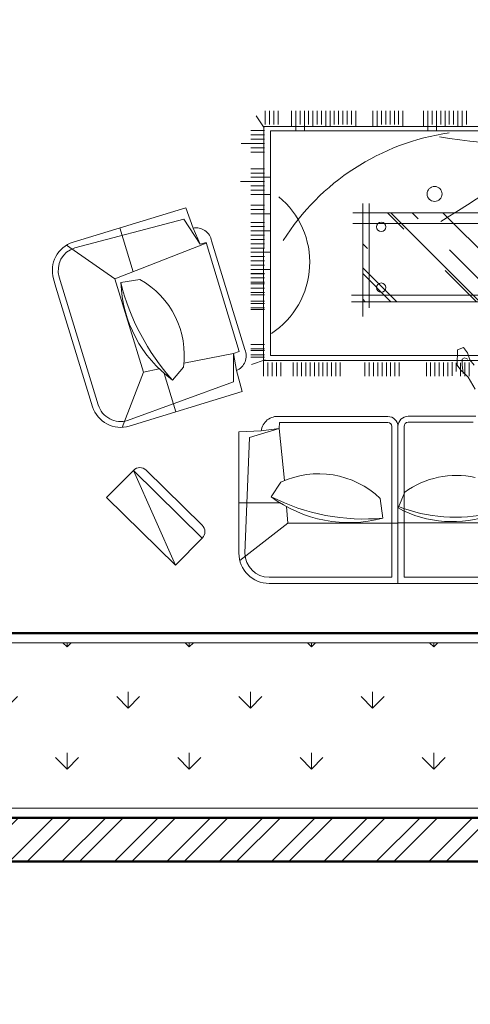
# Model space of a CAD drawing. Units: inches. Extents: x 261 to 2725, y 291 to 1454.
# Tile 29 of 35: x 2266 to 2359, y 467 to 670. Entities that reach past the tile are written whole.
import ezdxf

# ---------------------------------------------------------------- set-up
doc = ezdxf.new("R2010")
doc.units = ezdxf.units.IN
for name, color, linetype, lineweight in [('A-ANNO-DIMS', 136, 'Continuous', 18), ('A-FURN', 30, 'Continuous', 18), ('A-PLNT', 3, 'Continuous', 18), ('A-PLNT-PATT', 3, 'Continuous', 13), ('A-WALL', 222, 'Continuous', 50), ('A-WALL-PATT', 243, 'Continuous', 13)]:
    doc.layers.add(name, color=color, linetype=linetype, lineweight=lineweight)
doc.styles.get("Standard").update_dxf_attribs({"font": 'arial.ttf'})
doc.dimstyles.new('ISO-25', dxfattribs={"dimtxt": 12, "dimasz": 6, "dimexe": 1.25, "dimexo": 0.625, "dimtad": 1, "dimdec": 0, "dimlunit": 3, "dimtxsty": 'Standard', "dimblk": 'ARCHTICK', "dimcen": 2.5, "dimadec": 0, "dimazin": 0, "dimtfac": 1, "dimtdec": 0, "dimtmove": 0, "dimatfit": 3, "dimfxl": 1, "dimfxlon": 1, "dimarcsym": 0})

# ---------------------------------------------------------------- blocks, each defined once
blk = doc.blocks.new('A$C4DC51D13')
for p, q in [((3265.3, 2996.2), (1188.4, 2996.2)), ((1895.2, 2134), (1895.2, 2996.2)), ((1188.4, 2962.7), (1862.1, 2962.7)), ((1862.1, 2134), (1862.1, 2962.7)), ((1928.3, 2961.6), (2524.2, 2961.6)), ((1928.3, 2134), (1928.3, 2961.6)), ((296.4, 2525.2), (674.1, 2897)), ((443.7, 2375.5), (674.1, 2897)), ((674.1, 2897), (821.4, 2747.3)), ((1290.4, 2664.8), (1028, 2870.9)), ((1022.9, 2163.8), (1022.9, 2830.3)), ((1056, 2830.3), (1081, 2194.8)), ((443.7, 2375.5), (821.4, 2747.3)), ((820.9, 2676.6), (514.4, 2375)), ((1283.3, 2574.2), (1290.4, 2664.8)), ((1290.4, 2664.8), (1894.7, 2664.8)), ((1895.2, 2663.7), (2557.3, 2663.7)), ((1798, 2530.2), (1812.1, 2637.9)), ((1022.9, 2554.4), (1249.6, 2554.4)), ((1895.5, 2582.2), (1932.3, 2494.6)), ((443.7, 2375.5), (296.4, 2525.2)), ((1200, 2520.5), (1251.9, 2440.8)), ((1243.2, 2146.7), (1272.2, 2431.8)), ((1145.1, 2159.3), (1022.9, 2163.8)), ((1081, 2194.8), (1243.2, 2146.7)), ((498.8, 1837.1), (382.1, 2139.5)), ((1040.3, 1942.9), (421.2, 2132.6)), ((1145.1, 2159.3), (1243.2, 2146.7)), ((1244.8, 2113), (1243.2, 2146.7)), ((1839.5, 2113), (1244.8, 2113)), ((2308.5, 2111.9), (1950.4, 2111.9)), ((411.8, 2101.9), (992.6, 1890.2)), ((1839.5, 2079.9), (1244.8, 2079.9)), ((2322.1, 2078.8), (1950.4, 2078.8)), ((220.3, 2026), (19.3, 1370.1)), ((251.1, 2016.6), (37.1, 1314.7)), ((677.4, 2054.1), (612.9, 1843.6)), ((1009.7, 1828.1), (1040.3, 1942.9)), ((658.5, 1880), (717.8, 1809.1)), ((992.6, 1890.2), (993.4, 1733.4)), ((1158.3, 1784.3), (1158.3, 1858.2)), ((1181.8, 1784.3), (1181.8, 1858.2)), ((1205.3, 1784.3), (1205.3, 1858.2)), ((1228.8, 1784.3), (1228.8, 1858.2)), ((1252.2, 1784.3), (1252.2, 1858.2)), ((1319.4, 1784.3), (1319.4, 1858.2)), ((1342.9, 1784.3), (1342.9, 1858.2)), ((1366.3, 1784.3), (1366.3, 1858.2)), ((1389.8, 1784.3), (1389.8, 1858.2)), ((1413.3, 1784.3), (1413.3, 1858.2)), ((1436.8, 1784.3), (1436.8, 1858.2)), ((1460.2, 1784.3), (1460.2, 1858.2)), ((1483.7, 1784.3), (1483.7, 1858.2)), ((1507.2, 1784.3), (1507.2, 1858.2)), ((1530.7, 1784.3), (1530.7, 1858.2)), ((1554.1, 1784.3), (1554.1, 1858.2)), ((1577.6, 1784.3), (1577.6, 1858.2)), ((1714.2, 1784.3), (1714.2, 1858.2)), ((1737.6, 1784.3), (1737.6, 1858.2)), ((1761.1, 1784.3), (1761.1, 1858.2)), ((1784.6, 1784.3), (1784.6, 1858.2)), ((1808.1, 1784.3), (1808.1, 1858.2)), ((1831.5, 1784.3), (1831.5, 1858.2)), ((1855, 1784.3), (1855, 1858.2)), ((1878.5, 1784.3), (1878.5, 1858.2)), ((1902, 1784.3), (1902, 1858.2)), ((2050.7, 1784.3), (2050.7, 1858.2)), ((2074.2, 1784.3), (2074.2, 1858.2)), ((2097.7, 1784.3), (2097.7, 1858.2)), ((2121.1, 1784.3), (2121.1, 1858.2)), ((2144.6, 1784.3), (2144.6, 1858.2)), ((2168.1, 1784.3), (2168.1, 1858.2)), ((2191.6, 1782.4), (2191.6, 1856.3)), ((2238.5, 1785.1), (2238.5, 1859)), ((2262, 1784.3), (2262, 1858.2)), ((2285.4, 1784.3), (2285.4, 1858.2)), ((498.8, 1837.1), (341.4, 1323.6)), ((584.9, 1817.9), (498.8, 1837.1)), ((993.4, 1733.4), (720.4, 1787.6)), ((1009.7, 1828.1), (993.4, 1733.4)), ((1166.1, 1769.7), (1091.8, 1794.5)), ((1158.3, 1821.3), (1158.5, 487.7)), ((2215, 1785.7), (2215, 1832.3)), ((1024.2, 1722.3), (993.4, 1733.4)), ((1162.1, 1754.9), (1088.2, 1754.9)), ((1162.1, 1741.1), (1088.2, 1741.1)), ((3248.4, 1772.3), (1158.5, 1772.3)), ((1196, 511), (1196, 1744.8)), ((1196, 1744.8), (3215.6, 1744.8)), ((1024.2, 1722.3), (842.3, 1125.2)), ((873.1, 1115.8), (1055, 1712.9)), ((1162.1, 1717.6), (1088.2, 1717.6)), ((1162.1, 1708), (1088.2, 1708)), ((1162.1, 1684.5), (1088.2, 1684.5)), ((1701.7, 1530), (1701.7, 911.2)), ((1162.1, 1492.9), (1088.2, 1492.9)), ((1162.1, 1483.3), (1088.2, 1483.3)), ((1162.1, 1459.8), (1088.2, 1459.8)), ((1737.7, 1483.1), (1737.7, 911.2)), ((1162.1, 1446), (1088.2, 1446)), ((1162.1, 1412.8), (1088.2, 1412.8)), ((2674.6, 1449.9), (1641, 1449.9)), ((2674.6, 1413.9), (1641, 1413.9)), ((1888.1, 1449.9), (1701.7, 1263.5)), ((1856.2, 1449.9), (1701.7, 1295.4)), ((1715.1, 1449.9), (1701.7, 1436.5)), ((2343.3, 1449.9), (1855.3, 961.9)), ((2629.1, 1449), (2142, 961.9)), ((2325.1, 1449.9), (2154.2, 1279.1)), ((2461.6, 1449.9), (2177, 1165.3)), ((6.3, 1324.2), (19.3, 1370.2)), ((1162.1, 1399), (1088.2, 1399)), ((1162.1, 1375.5), (1088.2, 1375.5)), ((1162.1, 1352.1), (1088.2, 1352.1)), ((342.8, 1324.6), (76.7, 1139.6)), ((843, 1127.6), (342.8, 1324.6)), ((479.3, 1327.3), (375.2, 1344.9)), ((1162.1, 1342.9), (1088.2, 1342.9)), ((1162.1, 1342.4), (1088.2, 1342.4)), ((1162.1, 1319.4), (1088.2, 1319.4)), ((1162.1, 1318.9), (1088.2, 1318.9)), ((369.2, 1044.8), (442.9, 1285.2)), ((1162.1, 1296), (1088.2, 1296)), ((1162.1, 1295.5), (1088.2, 1295.5)), ((1196, 1272.5), (1088.2, 1272.5)), ((1162.1, 1272), (1088.2, 1272)), ((1162.1, 1249), (1088.2, 1249)), ((1162.1, 1248.5), (1088.2, 1248.5)), ((1162.1, 1225.5), (1088.2, 1225.5)), ((1162.1, 1202.1), (1088.2, 1202.1)), ((122.4, 1154.1), (719.7, 996.3)), ((1196, 1178.6), (1088.2, 1178.6)), ((1162.1, 1155.1), (1088.2, 1155.1)), ((1728.6, 1158.4), (1701.7, 1131.5)), ((732, 933.5), (112.9, 1123.3)), ((719.7, 996.3), (810.6, 1133.2)), ((771, 1045.7), (810.6, 1133.2)), ((842.3, 1125.2), (810.6, 1133.2)), ((1162.1, 1131.6), (1088.2, 1131.6)), ((1162.1, 1108.2), (1088.2, 1108.2)), ((1162.1, 1084.7), (1088.2, 1084.7)), ((771, 1045.7), (732, 933.5)), ((1196, 1061.2), (1088.2, 1061.2)), ((1162.1, 1037.7), (1088.2, 1037.7)), ((1926.6, 1051.5), (1837.1, 961.9)), ((1162.1, 1014.3), (1088.2, 1014.3)), ((1648.3, 1019.6), (2616.7, 1019.6)), ((2006.3, 994.6), (1973.6, 961.9)), ((1196, 967.3), (1088.2, 967.3)), ((1162.1, 943.8), (1088.2, 943.8)), ((1162.1, 920.4), (1088.2, 920.4)), ((1648.3, 961.9), (2681.9, 961.9)), ((1196, 860.5), (1088.2, 860.5)), ((1162.1, 837), (1088.2, 837)), ((1162.1, 813.5), (1088.2, 813.5)), ((1162.1, 790), (1031.8, 790)), ((1196, 766.6), (1088.2, 766.6)), ((1162.1, 743.1), (1088.2, 743.1)), ((1162.1, 719.6), (1088.2, 719.6)), ((1162.1, 627.8), (1088.2, 627.8)), ((1162.1, 604.4), (1088.2, 604.4)), ((1162.1, 580.9), (1034.2, 580.9)), ((1162.1, 557.4), (1088.2, 557.4)), ((1162.1, 533.9), (1088.2, 533.9)), ((1162.1, 510.5), (1088.2, 510.5)), ((1162, 495.1), (1116.6, 429)), ((1158.5, 487.7), (3248.4, 487.7)), ((3215.6, 511), (1196, 511)), ((1311.1, 487.7), (1311.1, 402.4)), ((1334.6, 511), (1334.6, 402.4)), ((1381.6, 511), (1381.6, 402.4)), ((1428.5, 487.7), (1428.5, 402.4)), ((1498.9, 487.7), (1498.9, 402.4)), ((1522.4, 487.7), (1522.4, 402.4)), ((1663.3, 487.7), (1663.3, 402.4)), ((1757.8, 487.7), (1757.8, 402.4)), ((1781.3, 487.7), (1781.3, 402.4)), ((1922.1, 487.7), (1922.1, 402.4)), ((2036, 487.7), (2036, 402.4)), ((2059.5, 511), (2059.5, 402.4)), ((2106.4, 511), (2106.4, 402.4)), ((2153.4, 487.7), (2153.4, 402.4)), ((2223.8, 487.7), (2223.8, 402.4)), ((2247.2, 487.7), (2247.2, 402.4)), ((1167.1, 476.3), (1167.1, 402.4)), ((1190.6, 476.3), (1190.6, 402.4)), ((1214, 476.3), (1214, 402.4)), ((1237.5, 476.3), (1237.5, 402.4)), ((1358.1, 476.3), (1358.1, 402.4)), ((1405, 476.3), (1405, 402.4)), ((1452, 476.3), (1452, 402.4)), ((1475.5, 476.3), (1475.5, 402.4)), ((1545.9, 476.3), (1545.9, 402.4)), ((1569.4, 476.3), (1569.4, 402.4)), ((1592.8, 476.3), (1592.8, 402.4)), ((1616.3, 476.3), (1616.3, 402.4)), ((1639.8, 476.3), (1639.8, 402.4)), ((1804.8, 476.3), (1804.8, 402.4)), ((1828.2, 476.3), (1828.2, 402.4)), ((1851.7, 476.3), (1851.7, 402.4)), ((1875.2, 476.3), (1875.2, 402.4)), ((1898.7, 476.3), (1898.7, 402.4)), ((2082.9, 476.3), (2082.9, 402.4)), ((2129.9, 476.3), (2129.9, 402.4)), ((2176.8, 476.3), (2176.8, 402.4)), ((2200.3, 476.3), (2200.3, 402.4)), ((2270.7, 476.3), (2270.7, 402.4))]:
    blk.add_line(p, q)
at = {"linetype": 'ByBlock'}
for points in [[(2319.3, 1929.9), (2280.8, 1863.6), (2257.7, 1842.4), (2239.2, 1825.7), (2220.1, 1798.2), (2221.6, 1713.1), (2254.3, 1700.7), (2275.9, 1729.8), (2288.6, 1768), (2313.7, 1797.6)], [(2279.2, 1765.9), (2259.2, 1757.4), (2247.6, 1764.7), (2246.4, 1796.2), (2253.5, 1843.5)]]:
    blk.add_lwpolyline(points, dxfattribs=at)
for centre, radius in [((1803.2, 1372.6), 25.7), ((1803.2, 1039.3), 25.7), ((2095.7, 858), 41)]:
    blk.add_circle(centre, radius)
for centre, radius, start, end in [((1188.4, 2830.3), 165.9, 90, 180), ((1188.4, 2830.3), 132.4, 90, 180), ((785.8, 2712.2), 50, 314.5497, 44.5497), ((1626.8, 1949.8), 712.7, 74.928, 126.7929), ((2192.2, 2032.6), 624.6, 69.4145, 118.3621), ((1707.9, 1527), 1115.8, 84.6406, 117.0804), ((2210.2, 1780.8), 852.5, 76.866, 111.6839), ((1459.9, 2882.7), 488.4, 244.7866, 313.8058), ((2216, 2892.1), 488.4, 234.4888, 282.1285), ((479.4, 2410.6), 50, 224.5497, 314.5497), ((374.1, 1978.9), 160.8, 72.9571, 162.9571), ((1234.5, 2169.3), 90, 186.4251, 276.5821), ((1839.5, 2135.1), 22.1, 270, 0), ((1839.5, 2135.1), 55.2, 270, 0), ((1950.4, 2134), 55.2, 180, 270), ((1950.4, 2134), 22.1, 180, 270), ((374.1, 1978.9), 128.6, 72.9571, 162.9571), ((1584.7, 1047), 1245.7, 138.0296, 166.1636), ((1067.1, 1321), 692.3, 126.1642, 178.0291), ((248.2, 1741.7), 474.4, 299.1514, 8.1705), ((974.8, 1747.9), 87.4, 336.375, 66.532), ((944.2, 1233.8), 467.1, 309.4804, 56.621), ((160.1, 1277), 160.8, 162.9571, 252.9571), ((160.1, 1277), 128.6, 162.9571, 252.9571), ((787.1, 1131.7), 87.4, 259.3822, 349.5393), ((2356.9, 1798.1), 1287.8, 212.1153, 261.9323), ((-29968.2, -49615.7), 59944, 56.743614, 57.623407), ((2591.9, -2109.1), 2694.5, 80.9842, 100.0261)]:
    blk.add_arc(centre, radius, start, end)
blk = doc.blocks.new('_ArchTick')
at = {"color": 0, "linetype": 'ByBlock', "const_width": 0.15}
blk.add_lwpolyline([(-0.5, -0.5), (0.5, 0.5)], dxfattribs=at)
blk = doc.blocks.new('*D71')
at = {"layer": 'A-ANNO-DIMS', "color": 0, "lineweight": -2, "ltscale": 0.07, "transparency": 16777216}
for p, q in [((2272.38, 690.06), (2272.38, 692.31)), ((2439.01, 690.06), (2439.01, 692.31)), ((2272.38, 691.06), (2439.01, 691.06)), ((2439.01, 691.06), (2725.34, 691.06))]:
    blk.add_line(p, q, dxfattribs=at)
at = {"layer": 'Defpoints', "color": 0, "ltscale": 0.07, "transparency": 16777216}
for p in [(2439.01, 691.06), (2272.38, 666.07), (2439.01, 666.07)]:
    blk.add_point(p, dxfattribs=at)
at = {"layer": 'A-ANNO-DIMS', "color": 0, "lineweight": -2, "ltscale": 0.07, "transparency": 16777216, "xscale": 6, "yscale": 6, "zscale": 6, "rotation": 180}
blk.add_blockref('_ArchTick', (2272.38, 691.06), dxfattribs=at)
at = {"layer": 'A-ANNO-DIMS', "color": 0, "lineweight": -2, "ltscale": 0.07, "transparency": 16777216, "xscale": 6, "yscale": 6, "zscale": 6}
blk.add_blockref('_ArchTick', (2439.01, 691.06), dxfattribs=at)
at = {"layer": 'A-ANNO-DIMS', "color": 0, "ltscale": 0.07, "transparency": 16777216, "insert": (2585.18, 697.9), "char_height": 12, "attachment_point": 5}
blk.add_mtext('TERRACE SEATING SET 13\'-10 1/2"', dxfattribs=at)
blk = doc.blocks.new('*D82')
at = {"layer": 'A-ANNO-DIMS', "color": 0, "lineweight": -2, "ltscale": 0.07, "transparency": 16777216}
for p, q in [((2600.96, 679.47), (2603.21, 679.47)), ((2601.96, 517.47), (2601.96, 679.47)), ((2600.96, 517.47), (2603.21, 517.47))]:
    blk.add_line(p, q, dxfattribs=at)
at = {"layer": 'Defpoints', "color": 0, "ltscale": 0.07, "transparency": 16777216}
for p in [(946.45, 679.47), (2601.96, 679.47), (946.45, 517.47)]:
    blk.add_point(p, dxfattribs=at)
at = {"layer": 'A-ANNO-DIMS', "color": 0, "lineweight": -2, "ltscale": 0.07, "transparency": 16777216, "xscale": 6, "yscale": 6, "zscale": 6}
for p, rotation in [((2601.96, 679.47), 90), ((2601.96, 517.47), 270)]:
    blk.add_blockref('_ArchTick', p, dxfattribs=dict(at, rotation=rotation))
at = {"layer": 'A-ANNO-DIMS', "color": 0, "ltscale": 0.07, "transparency": 16777216, "insert": (2595.2, 598.47), "char_height": 12, "attachment_point": 5, "rotation": 90}
blk.add_mtext('13\'-6"', dxfattribs=at)
blk = doc.blocks.new('*D89')
at = {"layer": 'A-ANNO-DIMS', "color": 0, "lineweight": -2, "ltscale": 0.07, "transparency": 16777216}
for p, q in [((2600.96, 508.47), (2603.21, 508.47)), ((2601.96, 412.47), (2601.96, 508.47)), ((2600.96, 412.47), (2603.21, 412.47))]:
    blk.add_line(p, q, dxfattribs=at)
at = {"layer": 'Defpoints', "color": 0, "ltscale": 0.07, "transparency": 16777216}
for p in [(955.45, 508.47), (2601.96, 508.47), (994.45, 412.47)]:
    blk.add_point(p, dxfattribs=at)
at = {"layer": 'A-ANNO-DIMS', "color": 0, "lineweight": -2, "ltscale": 0.07, "transparency": 16777216, "xscale": 6, "yscale": 6, "zscale": 6}
for p, rotation in [((2601.96, 508.47), 90), ((2601.96, 412.47), 270)]:
    blk.add_blockref('_ArchTick', p, dxfattribs=dict(at, rotation=rotation))
at = {"layer": 'A-ANNO-DIMS', "color": 0, "ltscale": 0.07, "transparency": 16777216, "insert": (2595.21, 460.47), "char_height": 12, "attachment_point": 5, "rotation": 90}
blk.add_mtext('8\'-0"', dxfattribs=at)
blk = doc.blocks.new('*D111')
at = {"layer": 'A-ANNO-DIMS', "color": 0, "lineweight": -2, "ltscale": 0.07, "transparency": 16777216}
for p, q in [((2600.96, 550.47), (2603.21, 550.47)), ((2601.96, 448.47), (2601.96, 550.47)), ((2600.96, 448.47), (2603.21, 448.47))]:
    blk.add_line(p, q, dxfattribs=at)
at = {"layer": 'Defpoints', "color": 0, "ltscale": 0.07, "transparency": 16777216}
for p in [(1720.08, 550.47), (2601.96, 550.47), (1720.08, 448.47)]:
    blk.add_point(p, dxfattribs=at)
at = {"layer": 'A-ANNO-DIMS', "color": 0, "lineweight": -2, "ltscale": 0.07, "transparency": 16777216, "xscale": 6, "yscale": 6, "zscale": 6}
for p, rotation in [((2601.96, 550.47), 90), ((2601.96, 448.47), 270)]:
    blk.add_blockref('_ArchTick', p, dxfattribs=dict(at, rotation=rotation))
at = {"layer": 'A-ANNO-DIMS', "color": 0, "ltscale": 0.07, "transparency": 16777216, "insert": (2595.21, 499.47), "char_height": 12, "attachment_point": 5, "rotation": 90}
blk.add_mtext('8\'-6"', dxfattribs=at)
blk = doc.blocks.new('*D112')
at = {"layer": 'A-ANNO-DIMS', "color": 0, "lineweight": -2, "ltscale": 0.07, "transparency": 16777216}
for p, q in [((2600.96, 679.47), (2603.21, 679.47)), ((2601.96, 550.47), (2601.96, 679.47)), ((2600.96, 550.47), (2603.21, 550.47))]:
    blk.add_line(p, q, dxfattribs=at)
at = {"layer": 'Defpoints', "color": 0, "ltscale": 0.07, "transparency": 16777216}
for p in [(1720.08, 679.47), (2601.96, 679.47), (1720.08, 550.47)]:
    blk.add_point(p, dxfattribs=at)
at = {"layer": 'A-ANNO-DIMS', "color": 0, "lineweight": -2, "ltscale": 0.07, "transparency": 16777216, "xscale": 6, "yscale": 6, "zscale": 6}
for p, rotation in [((2601.96, 679.47), 90), ((2601.96, 550.47), 270)]:
    blk.add_blockref('_ArchTick', p, dxfattribs=dict(at, rotation=rotation))
at = {"layer": 'A-ANNO-DIMS', "color": 0, "ltscale": 0.07, "transparency": 16777216, "insert": (2595.21, 614.97), "char_height": 12, "attachment_point": 5, "rotation": 90}
blk.add_mtext('10\'-9"', dxfattribs=at)
blk = doc.blocks.new('*D125')
at = {"layer": 'A-ANNO-DIMS', "color": 0, "lineweight": -2, "ltscale": 0.07, "transparency": 16777216}
for p, q in [((2600.96, 496.47), (2603.21, 496.47)), ((2601.96, 439.47), (2601.96, 496.47)), ((2600.96, 439.47), (2603.21, 439.47))]:
    blk.add_line(p, q, dxfattribs=at)
at = {"layer": 'Defpoints', "color": 0, "ltscale": 0.07, "transparency": 16777216}
for p in [(2214.67, 496.47), (2601.96, 496.47), (2214.67, 439.47)]:
    blk.add_point(p, dxfattribs=at)
at = {"layer": 'A-ANNO-DIMS', "color": 0, "lineweight": -2, "ltscale": 0.07, "transparency": 16777216, "xscale": 6, "yscale": 6, "zscale": 6}
for p, rotation in [((2601.96, 496.47), 90), ((2601.96, 439.47), 270)]:
    blk.add_blockref('_ArchTick', p, dxfattribs=dict(at, rotation=rotation))
at = {"layer": 'A-ANNO-DIMS', "color": 0, "ltscale": 0.07, "transparency": 16777216, "insert": (2595.21, 467.97), "char_height": 12, "attachment_point": 5, "rotation": 90}
blk.add_mtext('4\'-9"', dxfattribs=at)
blk = doc.blocks.new('*D136')
at = {"layer": 'A-ANNO-DIMS', "color": 0, "lineweight": -2, "ltscale": 0.07, "transparency": 16777216}
for p, q in [((2600.96, 675.78), (2603.21, 675.78)), ((2601.96, 675.78), (2601.96, 475.47)), ((2600.96, 475.47), (2603.21, 475.47))]:
    blk.add_line(p, q, dxfattribs=at)
at = {"layer": 'Defpoints', "color": 0, "ltscale": 0.07, "transparency": 16777216}
for p in [(2208.67, 675.78), (2208.67, 475.47), (2601.96, 475.47)]:
    blk.add_point(p, dxfattribs=at)
at = {"layer": 'A-ANNO-DIMS', "color": 0, "lineweight": -2, "ltscale": 0.07, "transparency": 16777216, "xscale": 6, "yscale": 6, "zscale": 6}
for p, rotation in [((2601.96, 675.78), 90), ((2601.96, 475.47), 270)]:
    blk.add_blockref('_ArchTick', p, dxfattribs=dict(at, rotation=rotation))
at = {"layer": 'A-ANNO-DIMS', "color": 0, "ltscale": 0.07, "transparency": 16777216, "insert": (2595.13, 575.62), "char_height": 12, "attachment_point": 5, "rotation": 90}
blk.add_mtext('16\'-8 1/2"', dxfattribs=at)
blk = doc.blocks.new('*D137')
at = {"layer": 'A-ANNO-DIMS', "color": 0, "lineweight": -2, "ltscale": 0.07, "transparency": 16777216}
for p, q in [((2600.96, 642.39), (2603.21, 642.39)), ((2601.96, 642.39), (2601.96, 634.05)), ((2600.96, 634.05), (2603.21, 634.05)), ((2601.96, 634.05), (2601.96, 566.94))]:
    blk.add_line(p, q, dxfattribs=at)
at = {"layer": 'Defpoints', "color": 0, "ltscale": 0.07, "transparency": 16777216}
for p in [(2221.19, 642.39), (2221.19, 634.05), (2601.96, 634.05)]:
    blk.add_point(p, dxfattribs=at)
at = {"layer": 'A-ANNO-DIMS', "color": 0, "lineweight": -2, "ltscale": 0.07, "transparency": 16777216, "xscale": 6, "yscale": 6, "zscale": 6}
for p, rotation in [((2601.96, 642.39), 90), ((2601.96, 634.05), 270)]:
    blk.add_blockref('_ArchTick', p, dxfattribs=dict(at, rotation=rotation))
at = {"layer": 'A-ANNO-DIMS', "color": 0, "ltscale": 0.07, "transparency": 16777216, "insert": (2595.13, 597.49), "char_height": 12, "attachment_point": 5, "rotation": 90}
blk.add_mtext('0\'-8 1/2"', dxfattribs=at)
blk = doc.blocks.new('*D138')
at = {"layer": 'A-ANNO-DIMS', "color": 0, "lineweight": -2, "ltscale": 0.07, "transparency": 16777216}
for p, q in [((2600.96, 634.05), (2603.21, 634.05)), ((2601.96, 634.05), (2601.96, 517.2)), ((2600.96, 517.2), (2603.21, 517.2))]:
    blk.add_line(p, q, dxfattribs=at)
at = {"layer": 'Defpoints', "color": 0, "ltscale": 0.07, "transparency": 16777216}
for p in [(2221.19, 634.05), (2221.19, 517.2), (2601.96, 517.2)]:
    blk.add_point(p, dxfattribs=at)
at = {"layer": 'A-ANNO-DIMS', "color": 0, "lineweight": -2, "ltscale": 0.07, "transparency": 16777216, "xscale": 6, "yscale": 6, "zscale": 6}
for p, rotation in [((2601.96, 634.05), 90), ((2601.96, 517.2), 270)]:
    blk.add_blockref('_ArchTick', p, dxfattribs=dict(at, rotation=rotation))
at = {"layer": 'A-ANNO-DIMS', "color": 0, "ltscale": 0.07, "transparency": 16777216, "insert": (2595.21, 575.62), "char_height": 12, "attachment_point": 5, "rotation": 90}
blk.add_mtext('9\'-9"', dxfattribs=at)

msp = doc.modelspace()

# ---------------------------------------------------------------- hatches: boundary and pattern name
at = {"layer": 'A-PLNT-PATT'}
h = msp.add_hatch(dxfattribs=at)
h.set_pattern_fill('GRASS', color=256, scale=0.7)
h.paths.add_polyline_path([(2052.71, 797.47), (2018.71, 797.47), (2018.71, 450.47), (2206.67, 450.47), (2206.67, 507.47), (2482.71, 507.47), (2482.71, 671.47), (2448.71, 671.47), (2448.71, 541.47), (2172.67, 541.47), (2172.67, 484.47), (2052.71, 484.47)])
at = {"layer": 'A-WALL-PATT'}
h = msp.add_hatch(dxfattribs=at)
h.set_pattern_fill('ANSI32', color=256, scale=0.8)
h.paths.add_polyline_path([(478.45, 685.47), (580.45, 685.47), (580.45, 691.47), (577.45, 691.47), (577.45, 694.47), (571.45, 694.47), (571.45, 691.47), (478.45, 691.47), (478.45, 721.47), (469.45, 721.47), (469.45, 508.47), (538.45, 508.47), (538.45, 517.47), (478.45, 517.47)])
h.paths.add_polyline_path([(694.45, 517.47), (676.45, 517.47), (676.45, 646.47), (670.45, 646.47), (670.45, 517.47), (610.45, 517.47), (610.45, 508.47), (694.45, 508.47)])
h.paths.add_polyline_path([(676.45, 784.47), (478.45, 784.47), (478.45, 844.47), (469.45, 844.47), (469.45, 745.47), (478.45, 745.47), (478.45, 775.47), (571.45, 775.47), (571.45, 724.47), (577.45, 724.47), (577.45, 775.47), (670.45, 775.47), (670.45, 691.47), (610.45, 691.47), (610.45, 685.47), (670.45, 685.47), (670.45, 682.47), (676.45, 682.47)])
h.paths.add_polyline_path([(955.45, 880.47), (946.45, 880.47), (946.45, 808.47), (778.45, 808.47), (778.45, 799.47), (946.45, 799.47), (946.45, 517.47), (898.45, 517.47), (898.45, 508.47), (955.45, 508.47)])
h.paths.add_polyline_path([(778.45, 598.47), (772.45, 598.47), (772.45, 517.47), (754.45, 517.47), (754.45, 508.47), (826.45, 508.47), (826.45, 517.47), (778.45, 517.47)])
h.paths.add_polyline_path([(955.45, 1090.47), (946.45, 1090.47), (946.45, 1030.47), (817.45, 1030.47), (817.45, 1024.47), (946.45, 1024.47), (946.45, 952.47), (955.45, 952.47)])
h.paths.add_polyline_path([(955.45, 1231.47), (730.45, 1231.47), (730.45, 1222.47), (772.45, 1222.47), (772.45, 1096.47), (766.45, 1096.47), (766.45, 1090.47), (772.45, 1090.47), (772.45, 1006.47), (712.45, 1006.47), (712.45, 1000.47), (778.45, 1000.47), (778.45, 1024.47), (781.45, 1024.47), (781.45, 1030.47), (778.45, 1030.47), (778.45, 1222.47), (946.45, 1222.47), (946.45, 1162.47), (955.45, 1162.47)])
h.paths.add_polyline_path([(694.45, 1231.47), (619.45, 1231.47), (619.45, 1222.47), (646.45, 1222.47), (646.45, 1039.47), (652.45, 1039.47), (652.45, 1090.47), (736.45, 1090.47), (736.45, 1096.47), (652.45, 1096.47), (652.45, 1222.47), (694.45, 1222.47)])
h.paths.add_polyline_path([(571.45, 1231.47), (469.45, 1231.47), (469.45, 1099.47), (478.45, 1099.47), (478.45, 1144.47), (544.45, 1144.47), (544.45, 1153.47), (538.45, 1153.47), (538.45, 1150.47), (478.45, 1150.47), (478.45, 1222.47), (538.45, 1222.47), (538.45, 1183.47), (544.45, 1183.47), (544.45, 1222.47), (571.45, 1222.47)])
h.paths.add_polyline_path([(538.45, 1006.47), (478.45, 1006.47), (478.45, 1051.47), (469.45, 1051.47), (469.45, 940.47), (478.45, 940.47), (478.45, 1000.47), (538.45, 1000.47)])
h.paths.add_polyline_path([(652.45, 1006.47), (652.45, 1009.47), (646.45, 1009.47), (646.45, 1006.47), (586.45, 1006.47), (586.45, 1000.47), (652.45, 1000.47)])
h.paths.add_polyline_path([(1288.08, 973.47), (1243.08, 973.47), (1243.08, 920.97), (1252.08, 920.97), (1252.08, 964.47), (1288.08, 964.47)], flags=17)
h.paths.add_polyline_path([(1402.08, 805.47), (1252.08, 805.47), (1252.08, 848.97), (1243.08, 848.97), (1243.08, 757.47), (1252.08, 757.47), (1252.08, 799.47), (1294.08, 799.47), (1372.08, 799.47), (1372.08, 779.47), (1372.08, 715.47), (1378.08, 715.47), (1378.08, 799.47), (1402.08, 799.47)])
h.paths.add_polyline_path([(1252.08, 721.47), (1243.08, 721.47), (1243.08, 439.47), (1729.08, 439.47), (1729.08, 709.47), (1720.08, 709.47), (1720.08, 679.47), (1582.08, 679.47), (1582.08, 670.47), (1588.08, 670.47), (1588.08, 673.47), (1720.08, 673.47), (1720.08, 559.47), (1690.08, 559.47), (1690.08, 550.47), (1720.08, 550.47), (1720.08, 448.47), (1252.08, 448.47), (1252.08, 496.47), (1312.08, 496.47), (1312.08, 505.47), (1252.08, 505.47), (1252.08, 673.47), (1405.08, 673.47), (1405.08, 679.47), (1378.08, 679.47), (1378.08, 685.47), (1372.08, 685.47), (1372.08, 679.47), (1252.08, 679.47)])
h.paths.add_polyline_path([(1450.08, 550.47), (1480.08, 550.47), (1480.08, 559.47), (1450.08, 559.47), (1450.08, 679.47), (1441.08, 679.47), (1441.08, 673.47), (1444.08, 673.47), (1444.08, 505.47), (1384.08, 505.47), (1384.08, 496.47), (1450.08, 496.47)], flags=17)
h.paths.add_polyline_path([(1618.08, 559.47), (1588.08, 559.47), (1588.08, 634.47), (1582.08, 634.47), (1582.08, 559.47), (1552.08, 559.47), (1552.08, 550.47), (1618.08, 550.47)], flags=17)
h.paths.add_polyline_path([(1564.08, 964.47), (1630.08, 964.47), (1630.08, 973.47), (1477.08, 973.47), (1477.08, 964.47), (1558.08, 964.47), (1558.08, 926.22), (1558.08, 887.97), (1486.08, 887.97), (1486.08, 881.97), (1558.08, 881.97), (1558.08, 805.47), (1450.08, 805.47), (1450.08, 845.97), (1444.08, 845.97), (1444.08, 805.47), (1438.08, 805.47), (1438.08, 799.47), (1564.08, 799.47)], flags=17)
h.paths.add_polyline_path([(1453.08, 973.47), (1408.08, 973.47), (1408.08, 964.47), (1444.08, 964.47), (1444.08, 881.97), (1450.08, 881.97), (1456.08, 881.97), (1456.08, 887.97), (1450.08, 887.97), (1450.08, 964.47), (1453.08, 964.47)], flags=17)
h.paths.add_polyline_path([(1729.08, 1231.47), (1243.08, 1231.47), (1243.08, 1167.47), (1252.08, 1167.47), (1252.08, 1222.47), (1441.08, 1222.47), (1441.08, 1045.47), (1648.08, 1045.47), (1648.08, 1051.47), (1450.08, 1051.47), (1450.08, 1074.47), (1450.08, 1222.47), (1472.08, 1222.47), (1720.08, 1222.47), (1720.08, 1051.47), (1708.08, 1051.47), (1708.08, 1045.47), (1720.08, 1045.47), (1720.08, 973.47), (1702.08, 973.47), (1702.08, 964.47), (1720.08, 964.47), (1720.08, 769.47), (1729.08, 769.47)])
h.paths.add_polyline_path([(2493.71, 1054.85), (2007.71, 1054.85), (2007.71, 439.47), (2214.67, 439.47), (2214.67, 496.47), (2493.71, 496.47)])
h.paths.add_polyline_path([(2016.71, 1045.85), (2304.71, 1045.85), (2304.71, 841.47), (2310.71, 841.47), (2310.71, 1045.85), (2484.71, 1045.85), (2484.71, 805.47), (2310.71, 805.47), (2310.71, 811.47), (2304.71, 811.47), (2304.71, 799.47), (2484.71, 799.47), (2484.71, 679.47), (2304.71, 679.47), (2304.71, 673.47), (2484.71, 673.47), (2484.71, 505.47), (2208.67, 505.47), (2208.67, 448.47), (2016.71, 448.47), (2016.71, 799.47), (2304.71, 799.47), (2304.71, 805.47), (2016.71, 805.47)], flags=16)

# ---------------------------------------------------------------- linework, layer by layer
at = {"layer": 'A-PLNT'}
for points in [[(2018.71, 797.47), (2018.71, 450.47), (2206.67, 450.47), (2206.67, 507.47), (2482.71, 507.47), (2482.71, 671.47)], [(2052.71, 797.47), (2052.71, 484.47), (2172.67, 484.47), (2172.67, 541.47), (2448.71, 541.47), (2448.71, 671.47)]]:
    msp.add_lwpolyline(points, dxfattribs=at)
at = {"layer": 'A-WALL'}
msp.add_line((2214.67, 496.47), (2493.71, 496.47), dxfattribs=at)
for points in [[(2016.71, 799.47), (2016.71, 448.47), (2208.67, 448.47), (2208.67, 505.47), (2484.71, 505.47), (2484.71, 673.47)], [(2054.71, 799.47), (2054.71, 486.47), (2170.67, 486.47), (2170.67, 543.47), (2446.71, 543.47), (2446.71, 673.47)]]:
    msp.add_lwpolyline(points, dxfattribs=at)

# ---------------------------------------------------------------- block references
at = {"layer": 'A-FURN', "xscale": -0.0374999999999198, "yscale": 0.0374999999999198, "zscale": 0.0374999999999198, "rotation": 180}
msp.add_blockref('A$C4DC51D13', (2272.61, 666.07), dxfattribs=at)

# ---------------------------------------------------------------- dimensions: what is measured, and where the dimension line sits
at = {"layer": 'A-ANNO-DIMS', "ltscale": 0.07}
dim = msp.add_linear_dim(base=(2439.01, 691.06), p1=(2272.38, 666.07), p2=(2439.01, 666.07), text='TERRACE SEATING SET <>', dimstyle='ISO-25', override={"dimdec": 1, "dimrnd": 0, "dimzin": 1, "dimlunit": 4, "dimfrac": 2}, dxfattribs=at)
dim.commit()
dim.dimension.update_dxf_attribs({"geometry": '*D71', "text_midpoint": (2585.18, 697.9)})
for base, p1, p2, picture, middle in [((2601.96, 679.47), (946.45, 517.47), (946.45, 679.47), '*D82', (2595.2, 598.47)), ((2601.96, 679.47), (1720.08, 550.47), (1720.08, 679.47), '*D112', (2595.21, 614.97)), ((2601.96, 475.47), (2208.67, 675.78), (2208.67, 475.47), '*D136', (2595.13, 575.62)), ((2601.96, 634.05), (2221.19, 642.39), (2221.19, 634.05), '*D137', (2595.13, 597.49)), ((2601.9578, 517.1998), (2221.1928, 634.0483), (2221.1928, 517.1998), '*D138', (2595.2059, 575.6241)), ((2601.96, 550.47), (1720.08, 448.47), (1720.08, 550.47), '*D111', (2595.21, 499.47)), ((2601.96, 508.47), (994.45, 412.47), (955.45, 508.47), '*D89', (2595.21, 460.47)), ((2601.96, 496.47), (2214.67, 439.47), (2214.67, 496.47), '*D125', (2595.21, 467.97))]:
    dim = msp.add_linear_dim(base=base, p1=p1, p2=p2, angle=90, dimstyle='ISO-25', override={"dimdec": 1, "dimlfac": 1, "dimrnd": 0, "dimzin": 1, "dimdsep": 46, "dimlunit": 4, "dimfrac": 2}, dxfattribs=at)
    dim.commit()
    dim.dimension.update_dxf_attribs({"geometry": picture, "text_midpoint": middle})

doc.saveas('drawing.dxf')
